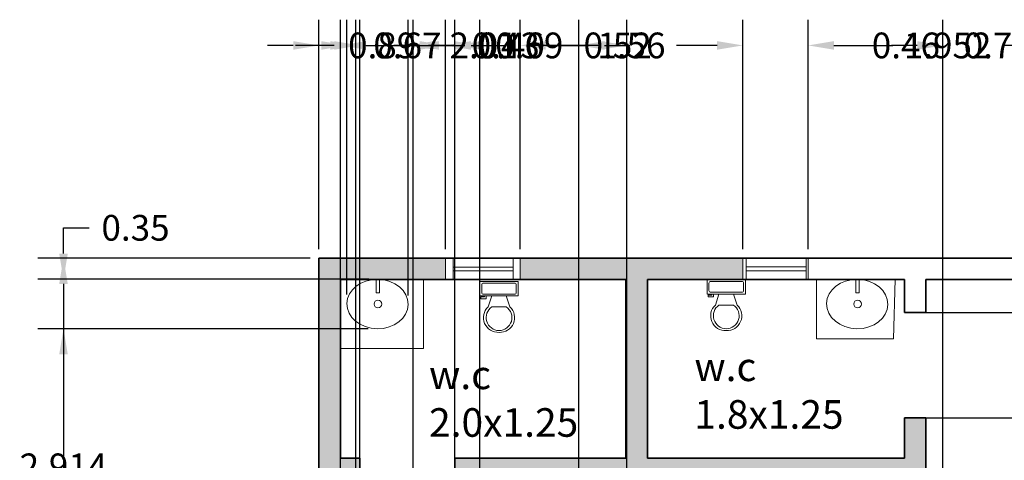
# Model space of a CAD drawing. Units: metres. Extents: x 36 to 56493, y 9 to 42849.
# Tile 4 of 5: x 56481.161 to 56488.056, y 42845.639 to 42848.722. Entities that reach past the tile are written whole.
import ezdxf

# ---------------------------------------------------------------- set-up
doc = ezdxf.new("R2010")
doc.units = ezdxf.units.M
doc.header["$MEASUREMENT"] = 0
for name, color, linetype, lineweight in [('A-ANNO-DIMS', 2, 'Continuous', 18), ('A-AREA-IDEN', 7, 'Continuous', 18), ('A-FLOR-FIXT', 8, 'Continuous', 18), ('A-GLAZ', 4, 'Continuous', 18), ('A-WALL', 7, 'Continuous', 35)]:
    doc.layers.add(name, color=color, linetype=linetype, lineweight=lineweight)
doc.layers.add('A-WALL-PATT', color=30, linetype='Continuous', lineweight=13, true_color=0xf26722)
doc.styles.get("Standard").update_dxf_attribs({"font": 'arial.ttf'})
doc.dimstyles.get("Standard").update_dxf_attribs({"dimtxt": 0.18, "dimasz": 0.18, "dimexe": 0.18, "dimexo": 0.0625, "dimgap": 0.09, "dimtad": 0, "dimtih": 1, "dimtoh": 1, "dimdec": 0, "dimzin": 0, "dimdsep": 46, "dimtxsty": 'Standard', "dimcen": 0.09, "dimadec": 0, "dimazin": 0, "dimtfac": 1, "dimtdec": 0, "dimtofl": 0, "dimtmove": 0, "dimatfit": 3, "dimfxl": 1, "dimtolj": 1, "dimtzin": 0, "dimarcsym": 0})

# ---------------------------------------------------------------- blocks, each defined once
blk = doc.blocks.new('*U2')
for p, q in [((9.5, -6), (9.5, -2)), ((-10, -8.5), (-8, -8.5)), ((-10, -9.5), (-10, -8.5)), ((-7, -9.5), (-10, -9.5)), ((-8, -8.5), (-8, -8)), ((-7, -8), (-7, -9.5)), ((-4, -8), (-6, -14)), ((4, -8), (6, -14)), ((4, -14), (-4, -14))]:
    blk.add_line(p, q)
blk.add_lwpolyline([(10.5, -8), (10.5, 0), (-10.5, 0), (-10.5, -8)], close=True)
for points in [[(-9.5, -2), (-9.5, -6)], [(8.5, -1), (-8.5, -1)], [(-8.5, -7), (8.5, -7)]]:
    blk.add_lwpolyline(points)
for centre, radius, start, end in [((-8.625, -1.875), 0.8839, 81.8699, 188.1301), ((8.625, -1.875), 0.8839, 351.8699, 98.1301), ((-8.625, -6.125), 0.8839, 171.869898, 278.1301), ((8.625, -6.125), 0.8839, 261.8699, 8.1301), ((-0.4772, -19.9188), 8.0953, 133.01722, 273.38), ((0.0374, -19.8731), 7.127, 124.50543, 269.7), ((-0.0373, -19.8731), 7.127, 270.3, 55.4946), ((0.4773, -19.9188), 8.0953, 266.62, 46.9828)]:
    blk.add_arc(centre, radius, start, end)
blk = doc.blocks.new('WASHBASIN-OVAL')
blk.add_lwpolyline([(0.2292, 0.3466), (0.2045, 0.3466), (0.2045, 0.2514), (0.2292, 0.2514)], close=True)
blk.add_circle((0.2168, 0.1733), 0.0268)
blk.add_ellipse((0.2144, 0.1733), major_axis=(0.2141, -0.003), ratio=0.809245)
blk = doc.blocks.new('*D18')
at = {"layer": 'A-ANNO-DIMS', "color": 0, "lineweight": -2, "transparency": 16777216}
for p, q in [((56483.1938, 42847.0533), (56481.2873, 42847.0533)), ((56481.4673, 42846.8733), (56481.4673, 42840.1703)), ((56481.4673, 42833.1033), (56481.4673, 42839.8063)), ((56483.1938, 42832.9233), (56481.2873, 42832.9233))]:
    blk.add_line(p, q, dxfattribs=at)
at = {"layer": 'A-ANNO-DIMS', "color": 0, "transparency": 16777216}
for points in [[(56481.4373, 42846.8733), (56481.4973, 42846.8733), (56481.4673, 42847.0533)], [(56481.4373, 42833.1033), (56481.4973, 42833.1033), (56481.4673, 42832.9233)]]:
    blk.add_solid(points, dxfattribs=at)
at = {"layer": 'Defpoints', "color": 0, "transparency": 16777216}
for p in [(56481.4673, 42847.0533), (56483.2563, 42847.0533), (56483.2563, 42832.9233)]:
    blk.add_point(p, dxfattribs=at)
at = {"layer": 'A-ANNO-DIMS', "color": 0, "transparency": 16777216, "insert": (56481.4673, 42839.9883), "char_height": 0.18, "attachment_point": 5}
blk.add_mtext('\\A1;14.13', dxfattribs=at)
blk = doc.blocks.new('*D25')
at = {"layer": 'A-ANNO-DIMS', "color": 0, "lineweight": -2, "transparency": 16777216}
for p, q in [((56483.5154, 42844.7198), (56483.5154, 42848.722)), ((56483.9169, 42844.7198), (56483.9169, 42848.722)), ((56483.3354, 42848.542), (56483.1554, 42848.542)), ((56484.0969, 42848.542), (56484.2769, 42848.542))]:
    blk.add_line(p, q, dxfattribs=at)
at = {"layer": 'A-ANNO-DIMS', "color": 0, "transparency": 16777216}
for points in [[(56483.3354, 42848.572), (56483.3354, 42848.512), (56483.5154, 42848.542)], [(56484.0969, 42848.572), (56484.0969, 42848.512), (56483.9169, 42848.542)]]:
    blk.add_solid(points, dxfattribs=at)
at = {"layer": 'Defpoints', "color": 0, "transparency": 16777216}
for p in [(56483.9169, 42848.542), (56483.5154, 42844.6573), (56483.9169, 42844.6573)]:
    blk.add_point(p, dxfattribs=at)
at = {"layer": 'A-ANNO-DIMS', "color": 0, "transparency": 16777216, "insert": (56484.6004, 42848.542), "char_height": 0.18, "attachment_point": 5}
blk.add_mtext('\\A1;0.40', dxfattribs=at)
blk = doc.blocks.new('*D31')
at = {"layer": 'A-ANNO-DIMS', "color": 0, "lineweight": -2, "transparency": 16777216}
for p, q in [((56483.452321, 42846.797813), (56483.452321, 42848.721953)), ((56483.880559, 42846.791872), (56483.880559, 42848.721953)), ((56483.272321, 42848.541953), (56483.092321, 42848.541953)), ((56484.060559, 42848.541953), (56484.240559, 42848.541953))]:
    blk.add_line(p, q, dxfattribs=at)
at = {"layer": 'A-ANNO-DIMS', "color": 0, "transparency": 16777216}
for points in [[(56483.272321, 42848.571953), (56483.272321, 42848.511953), (56483.452321, 42848.541953)], [(56484.060559, 42848.571953), (56484.060559, 42848.511953), (56483.880559, 42848.541953)]]:
    blk.add_solid(points, dxfattribs=at)
at = {"layer": 'Defpoints', "color": 0, "transparency": 16777216}
for p in [(56483.880559, 42848.541953), (56483.452321, 42846.735313), (56483.880559, 42846.729372)]:
    blk.add_point(p, dxfattribs=at)
at = {"layer": 'A-ANNO-DIMS', "color": 0, "transparency": 16777216, "insert": (56484.564338, 42848.541953), "char_height": 0.18, "attachment_point": 5}
blk.add_mtext('\\A1;0.43', dxfattribs=at)
blk = doc.blocks.new('*D32')
at = {"layer": 'A-ANNO-DIMS', "color": 0, "lineweight": -2, "transparency": 16777216}
for p, q in [((56481.4673, 42847.0856), (56481.4673, 42847.2656)), ((56481.4673, 42847.2656), (56481.6473, 42847.2656)), ((56483.6063, 42846.9056), (56481.2873, 42846.9056)), ((56483.6015, 42846.5591), (56481.2873, 42846.5591)), ((56481.4673, 42846.3791), (56481.4673, 42846.1991))]:
    blk.add_line(p, q, dxfattribs=at)
at = {"layer": 'A-ANNO-DIMS', "color": 0, "transparency": 16777216}
for points in [[(56481.4373, 42847.0856), (56481.4973, 42847.0856), (56481.4673, 42846.9056)], [(56481.4373, 42846.3791), (56481.4973, 42846.3791), (56481.4673, 42846.5591)]]:
    blk.add_solid(points, dxfattribs=at)
at = {"layer": 'Defpoints', "color": 0, "transparency": 16777216}
for p in [(56481.4673, 42846.9056), (56483.6688, 42846.9056), (56483.664, 42846.5591)]:
    blk.add_point(p, dxfattribs=at)
at = {"layer": 'A-ANNO-DIMS', "color": 0, "transparency": 16777216, "insert": (56481.9717, 42847.2656), "char_height": 0.18, "attachment_point": 5}
blk.add_mtext('\\A1;0.35', dxfattribs=at)
blk = doc.blocks.new('*D35')
at = {"layer": 'A-ANNO-DIMS', "color": 0, "lineweight": -2, "transparency": 16777216}
for p, q in [((56484.382516, 42839.15308), (56484.382516, 42848.721953)), ((56485.07636, 42839.15308), (56485.07636, 42848.721953)), ((56484.202516, 42848.541953), (56484.022516, 42848.541953)), ((56485.25636, 42848.541953), (56485.43636, 42848.541953))]:
    blk.add_line(p, q, dxfattribs=at)
at = {"layer": 'A-ANNO-DIMS', "color": 0, "transparency": 16777216}
for points in [[(56484.202516, 42848.571953), (56484.202516, 42848.511953), (56484.382516, 42848.541953)], [(56485.25636, 42848.571953), (56485.25636, 42848.511953), (56485.07636, 42848.541953)]]:
    blk.add_solid(points, dxfattribs=at)
at = {"layer": 'Defpoints', "color": 0, "transparency": 16777216}
for p in [(56485.07636, 42848.541953), (56484.382516, 42839.09058), (56485.07636, 42839.09058)]:
    blk.add_point(p, dxfattribs=at)
at = {"layer": 'A-ANNO-DIMS', "color": 0, "transparency": 16777216, "insert": (56484.729438, 42848.541953), "char_height": 0.18, "attachment_point": 5}
blk.add_mtext('\\A1;0.69', dxfattribs=at)
blk = doc.blocks.new('*D41')
at = {"layer": 'A-ANNO-DIMS', "color": 0, "lineweight": -2, "transparency": 16777216}
for p, q in [((56483.256252, 42847.115791), (56483.256252, 42848.721953)), ((56484.141772, 42847.115791), (56484.141772, 42848.721953)), ((56483.076252, 42848.541953), (56482.896252, 42848.541953)), ((56484.321772, 42848.541953), (56484.501772, 42848.541953))]:
    blk.add_line(p, q, dxfattribs=at)
at = {"layer": 'A-ANNO-DIMS', "color": 0, "transparency": 16777216}
for points in [[(56483.076252, 42848.571953), (56483.076252, 42848.511953), (56483.256252, 42848.541953)], [(56484.321772, 42848.571953), (56484.321772, 42848.511953), (56484.141772, 42848.541953)]]:
    blk.add_solid(points, dxfattribs=at)
at = {"layer": 'Defpoints', "color": 0, "transparency": 16777216}
for p in [(56484.141772, 42848.541953), (56483.256252, 42847.053291), (56484.141772, 42847.053291)]:
    blk.add_point(p, dxfattribs=at)
at = {"layer": 'A-ANNO-DIMS', "color": 0, "transparency": 16777216, "insert": (56483.699012, 42848.541953), "char_height": 0.18, "attachment_point": 5}
blk.add_mtext('\\A1;0.89', dxfattribs=at)
blk = doc.blocks.new('*D42')
at = {"layer": 'A-ANNO-DIMS', "color": 0, "lineweight": -2, "transparency": 16777216}
for p, q in [((56484.1418, 42847.1158), (56484.1418, 42848.722)), ((56484.665, 42847.1158), (56484.665, 42848.722)), ((56483.9618, 42848.542), (56483.7818, 42848.542)), ((56484.845, 42848.542), (56485.025, 42848.542))]:
    blk.add_line(p, q, dxfattribs=at)
at = {"layer": 'A-ANNO-DIMS', "color": 0, "transparency": 16777216}
for points in [[(56483.9618, 42848.572), (56483.9618, 42848.512), (56484.1418, 42848.542)], [(56484.845, 42848.572), (56484.845, 42848.512), (56484.665, 42848.542)]]:
    blk.add_solid(points, dxfattribs=at)
at = {"layer": 'Defpoints', "color": 0, "transparency": 16777216}
for p in [(56484.665, 42848.542), (56484.1418, 42847.0533), (56484.665, 42847.0533)]:
    blk.add_point(p, dxfattribs=at)
at = {"layer": 'A-ANNO-DIMS', "color": 0, "transparency": 16777216, "insert": (56485.3478, 42848.542), "char_height": 0.18, "attachment_point": 5}
blk.add_mtext('\\A1;0.52', dxfattribs=at)
blk = doc.blocks.new('*D43')
at = {"layer": 'A-ANNO-DIMS', "color": 0, "lineweight": -2, "transparency": 16777216}
for p, q in [((56484.665, 42847.1158), (56484.665, 42848.722)), ((56486.2245, 42847.1158), (56486.2245, 42848.722)), ((56484.845, 42848.542), (56485.1295, 42848.542)), ((56486.0445, 42848.542), (56485.76, 42848.542))]:
    blk.add_line(p, q, dxfattribs=at)
at = {"layer": 'A-ANNO-DIMS', "color": 0, "transparency": 16777216}
for points in [[(56484.845, 42848.572), (56484.845, 42848.512), (56484.665, 42848.542)], [(56486.0445, 42848.572), (56486.0445, 42848.512), (56486.2245, 42848.542)]]:
    blk.add_solid(points, dxfattribs=at)
at = {"layer": 'Defpoints', "color": 0, "transparency": 16777216}
for p in [(56486.2245, 42848.542), (56484.665, 42847.0533), (56486.2245, 42847.0533)]:
    blk.add_point(p, dxfattribs=at)
at = {"layer": 'A-ANNO-DIMS', "color": 0, "transparency": 16777216, "insert": (56485.4447, 42848.542), "char_height": 0.18, "attachment_point": 5}
blk.add_mtext('\\A1;1.56', dxfattribs=at)
blk = doc.blocks.new('*D44')
at = {"layer": 'A-ANNO-DIMS', "color": 0, "lineweight": -2, "transparency": 16777216}
for p, q in [((56486.2245, 42847.1158), (56486.2245, 42848.722)), ((56486.6826, 42847.1158), (56486.6826, 42848.722)), ((56486.0445, 42848.542), (56485.8645, 42848.542)), ((56486.8626, 42848.542), (56487.0426, 42848.542))]:
    blk.add_line(p, q, dxfattribs=at)
at = {"layer": 'A-ANNO-DIMS', "color": 0, "transparency": 16777216}
for points in [[(56486.0445, 42848.572), (56486.0445, 42848.512), (56486.2245, 42848.542)], [(56486.8626, 42848.572), (56486.8626, 42848.512), (56486.6826, 42848.542)]]:
    blk.add_solid(points, dxfattribs=at)
at = {"layer": 'Defpoints', "color": 0, "transparency": 16777216}
for p in [(56486.6826, 42848.542), (56486.2245, 42847.0533), (56486.6826, 42847.0533)]:
    blk.add_point(p, dxfattribs=at)
at = {"layer": 'A-ANNO-DIMS', "color": 0, "transparency": 16777216, "insert": (56487.3663, 42848.542), "char_height": 0.18, "attachment_point": 5}
blk.add_mtext('\\A1;0.46', dxfattribs=at)
blk = doc.blocks.new('*D45')
at = {"layer": 'A-ANNO-DIMS', "color": 0, "lineweight": -2, "transparency": 16777216}
for p, q in [((56486.6826, 42847.1158), (56486.6826, 42848.722)), ((56488.6347, 42847.1158), (56488.6347, 42848.722)), ((56486.8626, 42848.542), (56487.2744, 42848.542)), ((56488.4547, 42848.542), (56488.043, 42848.542))]:
    blk.add_line(p, q, dxfattribs=at)
at = {"layer": 'A-ANNO-DIMS', "color": 0, "transparency": 16777216}
for points in [[(56486.8626, 42848.572), (56486.8626, 42848.512), (56486.6826, 42848.542)], [(56488.4547, 42848.572), (56488.4547, 42848.512), (56488.6347, 42848.542)]]:
    blk.add_solid(points, dxfattribs=at)
at = {"layer": 'Defpoints', "color": 0, "transparency": 16777216}
for p in [(56488.6347, 42848.542), (56486.6826, 42847.0533), (56488.6347, 42847.0533)]:
    blk.add_point(p, dxfattribs=at)
at = {"layer": 'A-ANNO-DIMS', "color": 0, "transparency": 16777216, "insert": (56487.6587, 42848.542), "char_height": 0.18, "attachment_point": 5}
blk.add_mtext('\\A1;1.952', dxfattribs=at)
blk = doc.blocks.new('*D48')
at = {"layer": 'A-ANNO-DIMS', "color": 0, "lineweight": -2, "transparency": 16777216}
for p, q in [((56483.1938, 42847.0533), (56481.2873, 42847.0533)), ((56481.4673, 42846.8733), (56481.4673, 42845.7781)), ((56481.4673, 42844.3191), (56481.4673, 42845.4143)), ((56483.1938, 42844.1391), (56481.2873, 42844.1391))]:
    blk.add_line(p, q, dxfattribs=at)
at = {"layer": 'A-ANNO-DIMS', "color": 0, "transparency": 16777216}
for points in [[(56481.4373, 42846.8733), (56481.4973, 42846.8733), (56481.4673, 42847.0533)], [(56481.4373, 42844.3191), (56481.4973, 42844.3191), (56481.4673, 42844.1391)]]:
    blk.add_solid(points, dxfattribs=at)
at = {"layer": 'Defpoints', "color": 0, "transparency": 16777216}
for p in [(56483.2563, 42847.0533), (56481.4673, 42844.1391), (56483.2563, 42844.1391)]:
    blk.add_point(p, dxfattribs=at)
at = {"layer": 'A-ANNO-DIMS', "color": 0, "transparency": 16777216, "insert": (56481.4673, 42845.5962), "char_height": 0.18, "attachment_point": 5}
blk.add_mtext('\\A1;2.914', dxfattribs=at)
blk = doc.blocks.new('*D56')
at = {"layer": 'A-ANNO-DIMS', "color": 0, "lineweight": -2, "transparency": 16777216}
for p, q in [((56483.4063, 42842.9004), (56483.4063, 42848.722)), ((56485.4125, 42842.9004), (56485.4125, 42848.722)), ((56483.5863, 42848.542), (56484.1015, 42848.542)), ((56485.2325, 42848.542), (56484.7173, 42848.542))]:
    blk.add_line(p, q, dxfattribs=at)
at = {"layer": 'A-ANNO-DIMS', "color": 0, "transparency": 16777216}
for points in [[(56483.5863, 42848.572), (56483.5863, 42848.512), (56483.4063, 42848.542)], [(56485.2325, 42848.572), (56485.2325, 42848.512), (56485.4125, 42848.542)]]:
    blk.add_solid(points, dxfattribs=at)
at = {"layer": 'Defpoints', "color": 0, "transparency": 16777216}
for p in [(56485.4125, 42848.542), (56483.4063, 42842.8379), (56485.4125, 42842.8379)]:
    blk.add_point(p, dxfattribs=at)
at = {"layer": 'A-ANNO-DIMS', "color": 0, "transparency": 16777216, "insert": (56484.4094, 42848.542), "char_height": 0.18, "attachment_point": 5}
blk.add_mtext('\\A1;2.01', dxfattribs=at)
blk = doc.blocks.new('*D62')
at = {"layer": 'A-ANNO-DIMS', "color": 0, "lineweight": -2, "transparency": 16777216}
for p, q in [((56483.5429, 42845.5658), (56483.5429, 42848.722)), ((56484.2087, 42845.5658), (56484.2087, 42848.722)), ((56483.3629, 42848.542), (56483.1829, 42848.542)), ((56484.3887, 42848.542), (56484.5687, 42848.542))]:
    blk.add_line(p, q, dxfattribs=at)
at = {"layer": 'A-ANNO-DIMS', "color": 0, "transparency": 16777216}
for points in [[(56483.3629, 42848.572), (56483.3629, 42848.512), (56483.5429, 42848.542)], [(56484.3887, 42848.572), (56484.3887, 42848.512), (56484.2087, 42848.542)]]:
    blk.add_solid(points, dxfattribs=at)
at = {"layer": 'Defpoints', "color": 0, "transparency": 16777216}
for p in [(56484.2087, 42848.542), (56483.5429, 42845.5033), (56484.2087, 42845.5033)]:
    blk.add_point(p, dxfattribs=at)
at = {"layer": 'A-ANNO-DIMS', "color": 0, "transparency": 16777216, "insert": (56483.8758, 42848.542), "char_height": 0.18, "attachment_point": 5}
blk.add_mtext('\\A1;0.67', dxfattribs=at)
blk = doc.blocks.new('*D63')
at = {"layer": 'A-ANNO-DIMS', "color": 0, "lineweight": -2, "transparency": 16777216}
for p, q in [((56492.0308, 42846.6728), (56492.0308, 42846.8528)), ((56492.0308, 42846.8528), (56492.2108, 42846.8528)), ((56487.4188, 42846.6728), (56492.2108, 42846.6728)), ((56492.0308, 42846.1166), (56492.0308, 42846.4928)), ((56487.4188, 42845.9366), (56492.2108, 42845.9366))]:
    blk.add_line(p, q, dxfattribs=at)
at = {"layer": 'A-ANNO-DIMS', "color": 0, "transparency": 16777216}
for points in [[(56492.0008, 42846.4928), (56492.0608, 42846.4928), (56492.0308, 42846.6728)], [(56492.0008, 42846.1166), (56492.0608, 42846.1166), (56492.0308, 42845.9366)]]:
    blk.add_solid(points, dxfattribs=at)
at = {"layer": 'Defpoints', "color": 0, "transparency": 16777216}
for p in [(56487.3563, 42846.6728), (56492.0308, 42846.6728), (56487.3563, 42845.9366)]:
    blk.add_point(p, dxfattribs=at)
at = {"layer": 'A-ANNO-DIMS', "color": 0, "transparency": 16777216, "insert": (56492.5342, 42846.8528), "char_height": 0.18, "attachment_point": 5}
blk.add_mtext('\\A1;0.74', dxfattribs=at)
blk = doc.blocks.new('*D67')
at = {"layer": 'A-ANNO-DIMS', "color": 0, "lineweight": -2, "transparency": 16777216}
for p, q in [((56487.626252, 42839.785791), (56487.626252, 42848.721953)), ((56488.392626, 42839.785791), (56488.392626, 42848.721953)), ((56487.446252, 42848.541953), (56487.266252, 42848.541953)), ((56488.572626, 42848.541953), (56488.752626, 42848.541953))]:
    blk.add_line(p, q, dxfattribs=at)
at = {"layer": 'A-ANNO-DIMS', "color": 0, "transparency": 16777216}
for points in [[(56487.446252, 42848.571953), (56487.446252, 42848.511953), (56487.626252, 42848.541953)], [(56488.572626, 42848.571953), (56488.572626, 42848.511953), (56488.392626, 42848.541953)]]:
    blk.add_solid(points, dxfattribs=at)
at = {"layer": 'Defpoints', "color": 0, "transparency": 16777216}
for p in [(56488.392626, 42848.541953), (56487.626252, 42839.723291), (56488.392626, 42839.723291)]:
    blk.add_point(p, dxfattribs=at)
at = {"layer": 'A-ANNO-DIMS', "color": 0, "transparency": 16777216, "insert": (56488.009439, 42848.541953), "char_height": 0.18, "attachment_point": 5}
blk.add_mtext('\\A1;0.77', dxfattribs=at)

msp = doc.modelspace()

# ---------------------------------------------------------------- hatches: boundary and pattern name
at = {"layer": 'A-WALL-PATT'}
h = msp.add_hatch(color=256, dxfattribs=at)
h.dxf.hatch_style = 1
edge = h.paths.add_edge_path()
edge.add_line((56483.5429, 42845.6533), (56483.4063, 42845.6533))
edge.add_line((56483.4063, 42845.6533), (56483.4063, 42846.9033))
edge.add_line((56483.4063, 42846.9033), (56483.63, 42846.9033))
edge.add_ellipse((56483.6664, 42846.7323), major_axis=(0.2141, -0.003), ratio=0.809245, start_angle=94.07135, end_angle=102.818, ccw=False)
edge.add_line((56483.6565, 42846.9062), (56483.6565, 42846.9056))
edge.add_line((56483.6565, 42846.9056), (56483.6615, 42846.9056))
edge.add_ellipse((56483.6664, 42846.7323), major_axis=(0.2141, -0.003), ratio=0.809245, start_angle=90, end_angle=92.42655, ccw=False)
edge.add_line((56483.6812, 42846.9058), (56483.6812, 42846.9052))
edge.add_ellipse((56483.6664, 42846.7323), major_axis=(0.2141, -0.003), ratio=0.809245, start_angle=79.57494, end_angle=85.92601, ccw=False)
edge.add_line((56483.7048, 42846.9033), (56484.1418, 42846.9033))
edge.add_line((56484.1418, 42846.9033), (56484.1418, 42847.0533))
edge.add_line((56484.1418, 42847.0533), (56483.2563, 42847.0533))
edge.add_line((56483.2563, 42847.0533), (56483.2563, 42844.1391))
edge.add_line((56483.2563, 42844.1391), (56483.4063, 42844.1391))
edge.add_line((56483.4063, 42844.1391), (56483.4063, 42844.2368))
edge.add_line((56483.4063, 42844.2368), (56483.4063, 42845.5033))
edge.add_line((56483.4063, 42845.5033), (56483.5429, 42845.5033))
edge.add_line((56483.5429, 42845.5033), (56483.5429, 42845.6533))
edge = h.paths.add_edge_path(flags=0)
edge.add_line((56488.6347, 42847.0533), (56486.6826, 42847.0533))
edge.add_line((56486.6826, 42847.0533), (56486.6826, 42846.9033))
edge.add_line((56486.6826, 42846.9033), (56486.9892, 42846.9033))
edge.add_ellipse((56487.0257, 42846.7323), major_axis=(0.2141, -0.003), ratio=0.809245, start_angle=94.07135, end_angle=102.818, ccw=False)
edge.add_line((56487.0157, 42846.9062), (56487.0157, 42846.9056))
edge.add_line((56487.0157, 42846.9056), (56487.0207, 42846.9056))
edge.add_ellipse((56487.0257, 42846.7323), major_axis=(0.2141, -0.003), ratio=0.809245, start_angle=90, end_angle=92.42655, ccw=False)
edge.add_line((56487.0404, 42846.9058), (56487.0404, 42846.9052))
edge.add_ellipse((56487.0257, 42846.7323), major_axis=(0.2141, -0.003), ratio=0.809245, start_angle=79.57494, end_angle=85.92601, ccw=False)
edge.add_line((56487.064, 42846.9033), (56487.3563, 42846.9033))
edge.add_line((56487.3563, 42846.9033), (56487.3563, 42846.6728))
edge.add_line((56487.3563, 42846.6728), (56487.5063, 42846.6728))
edge.add_line((56487.5063, 42846.6728), (56487.5063, 42846.9033))
edge.add_line((56487.5063, 42846.9033), (56488.6347, 42846.9033))
edge.add_line((56488.6347, 42846.9033), (56488.6347, 42847.0533))
h.paths.add_polyline_path([(56486.2245, 42847.0533), (56484.665, 42847.0533), (56484.665, 42846.9033), (56485.4063, 42846.9033), (56485.4063, 42845.6533), (56484.2087, 42845.6533), (56484.2087, 42845.5033), (56487.3563, 42845.5033), (56487.3563, 42844.954), (56487.3563, 42843.021), (56487.5063, 42843.021), (56487.5063, 42843.2533), (56489.9401, 42843.2533), (56489.9401, 42843.4033), (56487.5063, 42843.4033), (56487.5063, 42845.6238), (56487.5063, 42845.6533), (56487.5063, 42845.9366), (56487.3563, 42845.9366), (56487.3563, 42845.6533), (56485.5563, 42845.6533), (56485.5563, 42846.9033), (56486.2245, 42846.9033)])
h.paths.add_polyline_path([(56491.1563, 42847.0533), (56489.9198, 42847.0533), (56489.9198, 42846.9033), (56489.9717, 42846.9033), (56491.0063, 42846.9033), (56491.0063, 42845.887), (56491.1563, 42845.887)])
h.paths.add_polyline_path([(56491.1563, 42844.3264), (56491.0063, 42844.3264), (56491.0063, 42843.4033), (56490.7805, 42843.4033), (56490.7805, 42843.2533), (56491.0063, 42843.2533), (56491.0063, 42839.8733), (56488.3926, 42839.8733), (56488.3926, 42839.7233), (56491.0063, 42839.7233), (56491.0063, 42836.1233), (56487.6263, 42836.1233), (56487.6263, 42839.0009), (56487.4763, 42839.0009), (56487.4763, 42836.1233), (56486.4863, 42836.1233), (56486.4863, 42835.9733), (56487.4763, 42835.9733), (56487.8849, 42835.9733), (56487.8849, 42832.9233), (56487.8913, 42832.9233), (56488.0349, 42832.9233), (56488.0349, 42833.0733), (56488.0349, 42835.9733), (56491.0063, 42835.9733), (56491.0063, 42833.0733), (56491.0063, 42832.9233), (56491.1563, 42832.9233), (56491.1563, 42835.9733)])
h.paths.add_polyline_path([(56483.4063, 42842.8378), (56483.2563, 42842.8378), (56483.2563, 42841.5433), (56483.2563, 42840.8898), (56483.4063, 42840.8898), (56483.4063, 42841.3933), (56485.0063, 42841.3933), (56485.0063, 42841.2426), (56485.1563, 42841.2426), (56485.1563, 42841.3933), (56487.3563, 42841.3933), (56487.5063, 42841.3933), (56487.5063, 42841.9264), (56487.3563, 42841.9264), (56487.3563, 42841.5433), (56483.4063, 42841.5433)])
h.paths.add_polyline_path([(56485.1563, 42840.351), (56485.0063, 42840.351), (56485.0063, 42839.8933), (56483.4063, 42839.8933), (56483.4063, 42840.3779), (56483.2563, 42840.3779), (56483.2563, 42839.8933), (56483.2563, 42838.6997), (56483.4063, 42838.6997), (56483.4063, 42839.7433), (56485.1563, 42839.7433)])
h.paths.add_polyline_path([(56483.4063, 42836.7612), (56483.2563, 42836.7612), (56483.2563, 42835.6733), (56483.2563, 42834.2533), (56483.2563, 42832.9233), (56485.9871, 42832.9233), (56485.9871, 42833.0733), (56483.4063, 42833.0733), (56483.4063, 42834.2533), (56483.4063, 42835.5233), (56485.4763, 42835.5233), (56485.9871, 42835.5233), (56485.9871, 42835.6733), (56485.6263, 42835.6733), (56483.4063, 42835.6733)])

# ---------------------------------------------------------------- linework, layer by layer
at = {"layer": 'A-FLOR-FIXT'}
for p, q in [((56483.9883, 42846.9033), (56483.9883, 42846.4218)), ((56486.7408, 42846.9033), (56486.7408, 42846.4878)), ((56487.2798, 42846.4878), (56487.2912, 42846.9033)), ((56486.7408, 42846.4878), (56487.2798, 42846.4878)), ((56483.9883, 42846.4218), (56483.4063, 42846.4218))]:
    msp.add_line(p, q, dxfattribs=at)
at = {"layer": 'A-GLAZ'}
for p, q in [((56484.1418, 42847.0533), (56484.1418, 42846.9033)), ((56484.1963, 42846.9033), (56484.1963, 42847.0533)), ((56484.1963, 42846.9901), (56484.6163, 42846.9901)), ((56484.6163, 42846.9033), (56484.6163, 42847.0533)), ((56484.665, 42847.0533), (56484.665, 42846.9033)), ((56486.2245, 42847.0533), (56486.2245, 42846.9033)), ((56486.2472, 42847.0533), (56486.2472, 42846.9033)), ((56486.2472, 42846.9914), (56486.6672, 42846.9914)), ((56486.6672, 42847.0533), (56486.6672, 42846.9033)), ((56486.6826, 42847.0533), (56486.6826, 42846.9033)), ((56484.1963, 42846.9651), (56484.6163, 42846.9651)), ((56486.2472, 42846.9641), (56486.6672, 42846.9641)), ((56484.1418, 42846.9033), (56484.1418, 42846.9033))]:
    msp.add_line(p, q, dxfattribs=at)
at = {"layer": 'A-WALL'}
for p, q in [((56483.2563, 42847.0533), (56485.4063, 42847.0533)), ((56483.2563, 42834.2533), (56483.2563, 42847.0533)), ((56483.2563, 42847.0533), (56491.1563, 42847.0533)), ((56485.5563, 42847.0533), (56487.3563, 42847.0533)), ((56483.4063, 42846.9033), (56485.4063, 42846.9033)), ((56483.4063, 42845.6533), (56483.4063, 42846.9033)), ((56485.4063, 42846.9033), (56485.4063, 42845.6533)), ((56485.5563, 42846.9033), (56485.5563, 42845.6533)), ((56485.5563, 42846.9033), (56487.3563, 42846.9033)), ((56487.3563, 42846.9033), (56487.3563, 42846.6728)), ((56487.5063, 42846.9033), (56487.5063, 42846.6728)), ((56487.5063, 42846.9033), (56491.0063, 42846.9033)), ((56487.3563, 42846.6728), (56487.5063, 42846.6728)), ((56487.3563, 42845.9366), (56487.5063, 42845.9366)), ((56487.3563, 42845.9366), (56487.3563, 42845.6533)), ((56487.5063, 42845.9366), (56487.5063, 42845.6533)), ((56483.5429, 42845.6533), (56483.4063, 42845.6533)), ((56483.5429, 42845.6533), (56483.5429, 42845.5033)), ((56485.4063, 42845.6533), (56484.2087, 42845.6533)), ((56484.2087, 42845.6533), (56484.2087, 42845.5033)), ((56487.3563, 42845.6533), (56485.5563, 42845.6533)), ((56487.5063, 42843.4033), (56487.5063, 42845.6533))]:
    msp.add_line(p, q, dxfattribs=at)

# ---------------------------------------------------------------- block references
at = {"layer": 'A-FLOR-FIXT'}
for p in [(56483.452, 42846.559), (56486.8112, 42846.559)]:
    msp.add_blockref('WASHBASIN-OVAL', p, dxfattribs=at)
at = {"layer": 'A-FLOR-FIXT', "xscale": 0.0127360389341166, "yscale": 0.0127360389341166, "zscale": 0.0127360389341166}
for p in [(56484.5174, 42846.8906), (56486.1085, 42846.9033)]:
    msp.add_blockref('*U2', p, dxfattribs=at)

# ---------------------------------------------------------------- texts
at = {"layer": 'A-AREA-IDEN', "char_height": 0.2, "attachment_point": 1}
for s, insert in [('w.c\\P1.8x1.25', (56485.8854, 42846.3929)), ('w.c\\P2.0x1.25', (56484.0273, 42846.3366))]:
    msp.add_mtext_dynamic_manual_height_columns(s, width=0.817901, gutter_width=1, heights=[0], dxfattribs=dict(at, insert=insert))

# ---------------------------------------------------------------- dimensions: what is measured, and where the dimension line sits
at = {"layer": 'A-ANNO-DIMS'}
for base, p1, p2, override, picture, middle in [((56484.1418, 42848.542), (56483.2563, 42847.0533), (56484.1418, 42847.0533), {"dimdec": 2, "dimlfac": 1, "dimrnd": 0, "dimzin": 0, "dimdsep": 46, "dimlunit": 2}, '*D41', (56483.699, 42848.542)), ((56483.8806, 42848.542), (56483.4523, 42846.7353), (56483.8806, 42846.7294), {"dimdec": 2, "dimlfac": 1, "dimrnd": 0, "dimzin": 0, "dimdsep": 46, "dimlunit": 2}, '*D31', (56484.5643, 42848.542)), ((56483.9169, 42848.542), (56483.5154, 42844.6573), (56483.9169, 42844.6573), {"dimdec": 2, "dimlfac": 1, "dimrnd": 0, "dimzin": 0, "dimdsep": 46, "dimlunit": 2}, '*D25', (56484.6004, 42848.542)), ((56484.2087, 42848.542), (56483.5429, 42845.5033), (56484.2087, 42845.5033), {"dimdec": 2, "dimlfac": 1, "dimrnd": 0, "dimzin": 0, "dimdsep": 46, "dimlunit": 2}, '*D62', (56483.8758, 42848.542)), ((56485.4125, 42848.542), (56483.4063, 42842.8378), (56485.4125, 42842.8378), {"dimdec": 2, "dimlfac": 1, "dimrnd": 0, "dimzin": 0, "dimdsep": 46, "dimlunit": 2}, '*D56', (56484.4094, 42848.542)), ((56484.665, 42848.542), (56484.1418, 42847.0533), (56484.665, 42847.0533), {"dimdec": 2, "dimlfac": 1, "dimrnd": 0, "dimzin": 0, "dimdsep": 46, "dimlunit": 2}, '*D42', (56485.3478, 42848.542)), ((56485.0764, 42848.542), (56484.3825, 42839.0906), (56485.0764, 42839.0906), {"dimdec": 2, "dimlfac": 1, "dimrnd": 0, "dimzin": 0, "dimdsep": 46, "dimlunit": 2}, '*D35', (56484.7294, 42848.542)), ((56486.2245, 42848.542), (56484.665, 42847.0533), (56486.2245, 42847.0533), {"dimdec": 2, "dimlfac": 1, "dimrnd": 0, "dimzin": 0, "dimdsep": 46, "dimlunit": 2}, '*D43', (56485.4447, 42848.542)), ((56486.6826, 42848.542), (56486.2245, 42847.0533), (56486.6826, 42847.0533), {"dimdec": 2, "dimlfac": 1, "dimrnd": 0, "dimzin": 0, "dimdsep": 46, "dimlunit": 2}, '*D44', (56487.3663, 42848.542)), ((56488.6347, 42848.542), (56486.6826, 42847.0533), (56488.6347, 42847.0533), {"dimdec": 3, "dimlfac": 1, "dimrnd": 0, "dimzin": 0, "dimdsep": 46, "dimlunit": 2}, '*D45', (56487.6587, 42848.542)), ((56488.3926, 42848.542), (56487.6263, 42839.7233), (56488.3926, 42839.7233), {"dimdec": 2, "dimlfac": 1, "dimrnd": 0, "dimzin": 0, "dimdsep": 46, "dimlunit": 2}, '*D67', (56488.0094, 42848.542))]:
    dim = msp.add_linear_dim(base=base, p1=p1, p2=p2, dimstyle='Standard', override=override, dxfattribs=at)
    dim.commit()
    dim.dimension.update_dxf_attribs({"geometry": picture, "text_midpoint": middle})
for base, p1, p2, override, picture, middle in [((56481.4673, 42846.9056), (56483.664, 42846.5591), (56483.6688, 42846.9056), {"dimdec": 2, "dimlfac": 1, "dimrnd": 0, "dimzin": 0, "dimdsep": 46, "dimlunit": 2}, '*D32', (56481.9717, 42847.2656)), ((56481.4673, 42847.0533), (56483.2563, 42832.9233), (56483.2563, 42847.0533), {"dimdec": 2, "dimlfac": 1, "dimrnd": 0, "dimzin": 0, "dimdsep": 46, "dimlunit": 2}, '*D18', (56481.4673, 42839.9883)), ((56481.4673, 42844.1391), (56483.2563, 42847.0533), (56483.2563, 42844.1391), {"dimdec": 3, "dimlfac": 1, "dimrnd": 0, "dimzin": 0, "dimdsep": 46, "dimlunit": 2}, '*D48', (56481.4673, 42845.5962)), ((56492.0308, 42846.6728), (56487.3563, 42845.9366), (56487.3563, 42846.6728), {"dimdec": 2, "dimlfac": 1, "dimrnd": 0, "dimzin": 0, "dimdsep": 46, "dimlunit": 2}, '*D63', (56492.5342, 42846.8528))]:
    dim = msp.add_linear_dim(base=base, p1=p1, p2=p2, angle=90, dimstyle='Standard', override=override, dxfattribs=at)
    dim.commit()
    dim.dimension.update_dxf_attribs({"geometry": picture, "text_midpoint": middle})

doc.saveas('drawing.dxf')
